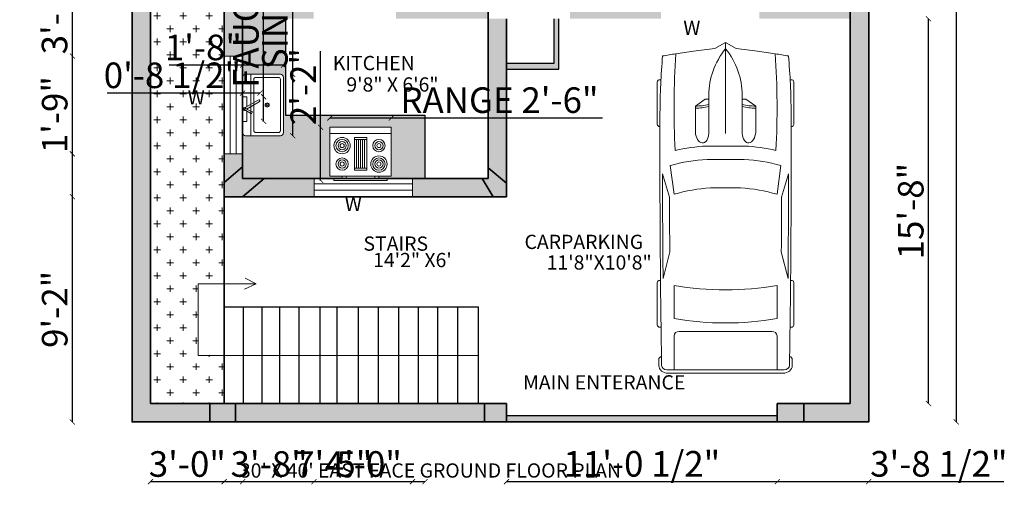
# Model space of a CAD drawing. Units: inches. Extents: x 1858 to 2399, y 1317 to 1943.
# Tile 1 of 8: x 1858 to 2340, y 1317 to 1554. Entities that reach past the tile are written whole.
import ezdxf

# ---------------------------------------------------------------- set-up
doc = ezdxf.new("R2010")
doc.units = ezdxf.units.IN
for name, color, linetype, lineweight in [('A-ANNO-DIMS', 2, 'Continuous', 18), ('A-ANNO-SYMB', 7, 'Continuous', 18), ('A-ANNO-TEXT', 7, 'Continuous', 18), ('A-AREA-IDEN', 7, 'Continuous', 18), ('A-COLS', 7, 'Continuous', 35), ('A-COLS-PATT', 5, 'Continuous', 13), ('A-DOOR', 4, 'Continuous', 25), ('A-EQPM', 8, 'Continuous', 18), ('A-EQPM-VEHI', 8, 'Continuous', 18), ('A-FLOR-CASE', 8, 'Continuous', 25), ('A-FLOR-FIXT', 9, 'Continuous', 18), ('A-FLOR-FIXT-PATT', 9, 'Continuous', 13), ('A-WALL', 7, 'Continuous', 35), ('A-WALL-PATT', 1, 'Continuous', 13), ('L-SITE-PATT', 8, 'Continuous', 13), ('stairs', 3, 'Continuous', 25), ('window', 4, 'Continuous', 18)]:
    doc.layers.add(name, color=color, linetype=linetype, lineweight=lineweight)
doc.styles.get("Standard").update_dxf_attribs({"font": 'arial.ttf'})
doc.dimstyles.new('ISO-25', dxfattribs={"dimtxt": 12.5, "dimasz": 2.5, "dimexe": 1.25, "dimexo": 0.625, "dimtad": 1, "dimdec": 0, "dimlunit": 4, "dimtxsty": 'Standard', "dimblk": 'ARCHTICK', "dimcen": 2.5, "dimse1": 1, "dimse2": 1, "dimclrd": 3, "dimclrt": 4, "dimadec": 0, "dimazin": 0, "dimtfac": 1, "dimtdec": 0, "dimtmove": 0, "dimatfit": 3, "dimfxl": 1, "dimarcsym": 0})

# ---------------------------------------------------------------- blocks, each defined once
blk = doc.blocks.new('*U6')
for p, q in [((21.1, 37.41), (21.1, 36.83)), ((46.55, 38.89), (22.35, 38.89)), ((47.8, 37.39), (47.8, 37.41)), ((87.99, 31.87), (74.76, 35.92)), ((134.31, 35.6), (119.29, 31.78)), ((135.45, 37.07), (135.45, 37.41)), ((136.7, 38.89), (160.9, 38.89)), ((162.15, 37.41), (162.15, 36.77)), ((70.03, 31.54), (86.41, 29.35)), ((138.42, 29.35), (157.25, 29.35)), ((186.47, 29.35), (167.01, 29.35)), ((186.47, -33.5), (186.47, 33.5)), ((188.4, -32.76), (188.4, 32.76)), ((164.52, 26.39), (164.52, -26.39)), ((32.27, 11.63), (36.13, 17.17)), ((36.13, 17.17), (50.94, 17.17)), ((3.27, 6.13), (0.1, 0.41)), ((29.77, 9.51), (51.68, 9.51)), ((32.12, 9.51), (32.12, 11.15)), ((58.92, -10.77), (58.92, 10.77)), ((66.55, -10.53), (66.55, 10.53)), ((82.74, 8.5), (82.74, -8.5)), ((186.47, -10.53), (186.47, 10.53)), ((0, 0), (51.68, 0)), ((0.1, -0.41), (3.27, -6.13)), ((29.77, -9.51), (51.68, -9.51)), ((32.12, -9.51), (32.12, -11.15)), ((32.27, -11.63), (36.13, -17.17)), ((36.13, -17.17), (50.94, -17.17)), ((86.41, -29.35), (70.03, -31.54)), ((87.99, -31.87), (74.76, -35.92)), ((134.31, -35.6), (119.29, -31.78)), ((157.25, -29.35), (138.42, -29.35)), ((167.01, -29.35), (186.47, -29.35)), ((21.1, -37.41), (21.1, -36.83)), ((46.55, -38.89), (22.35, -38.89)), ((47.8, -37.39), (47.8, -37.41)), ((135.45, -37.07), (135.45, -37.41)), ((136.7, -38.89), (160.9, -38.89)), ((162.15, -37.41), (162.15, -36.77))]:
    blk.add_line(p, q)
for centre, major_axis, ratio, start_param, end_param in [((266.03, -27.52), (0, 313.31), 0.842304, 1.367076, 1.39176), ((41.19, -490.86), (0, 528.23), 0.842304, 0.00281, 0.075598), ((22.35, 37.41), (0, -1.48), 0.842304, 3.141593, 4.712389), ((64.48, -10555.62), (0, 10593.03), 0.842304, -0.013397, 0.002797), ((46.55, 37.41), (0, 1.48), 0.842304, -1.570796, 0), ((64.48, -10555.62), (0, -10591.55), 0.842304, 3.133765, 3.140441), ((136.7, 37.41), (0, -1.48), 0.842304, 3.141593, 4.712389), ((160.9, 37.41), (0, 1.48), 0.842304, -1.570796, 0), ((180.63, 35.84), (0, 2.22), 0.842304, -0.013017, 1.249894), ((64.48, -10556.36), (0, 10595.31), 0.842304, -0.013397, -0.013017), ((183.98, 33.5), (0, -2.96), 0.842304, 1.570796, 3.128196), ((183.98, 32.76), (0, -5.25), 0.842304, 1.570796, 3.128196), ((259.18, -27.52), (0, -305.3), 0.842304, 4.528606, 4.561838), ((37.47, -593.96), (0, -623.33), 0.842304, 3.096046, 3.200911), ((134.4, 5.39), (0, -89.78), 0.842304, 4.449482, 4.652344), ((135.29, 5.39), (0, 81.77), 0.842304, 1.245306, 1.50788), ((149.6, 2.8), (0, -79.58), 0.842304, 4.372215, 4.640744), ((95.79, -3666.35), (0, -3698.24), 0.842304, 3.134049, 3.144098), ((17.08, 0), (0, 147.02), 0.842304, 4.511394, 4.913384), ((35.91, 0), (0, 147.02), 0.842304, 4.511394, 4.913384), ((167.01, 26.39), (0, 2.96), 0.842304, 0, 1.570796), ((-204.49, 52.4), (0, -250.96), 0.842304, 1.385369, 1.434372), ((13.04, 17.01), (0, 27.42), 0.842304, 4.435146, 4.718221), ((14.2, 17.01), (0, 27.42), 0.842304, 4.435146, 4.718221), ((50.79, 13.34), (6.34, -0.36), 0.603834, -1.395552, 1.581315), ((32.75, 11.15), (0, 0.74), 0.842304, 0.879714, 1.570796), ((29.77, -46.66), (0, 56.17), 0.842304, 0, 0.590319), ((0.62, 0), (0, -0.74), 0.842304, 4.131459, 5.293319), ((29.77, 46.66), (0, 56.17), 0.842304, 2.551274, 3.141593), ((-204.49, -52.4), (0, 250.96), 0.842304, -1.434372, -1.385369), ((32.75, -11.15), (0, -0.74), 0.842304, 4.712389, 5.403472), ((13.04, -17.01), (0, -27.42), 0.842304, 1.564964, 1.848039), ((14.2, -17.01), (0, -27.42), 0.842304, 1.564964, 1.848039), ((134.4, -5.39), (0, -89.78), 0.842304, -1.510751, -1.307889), ((135.29, -5.39), (0, -81.77), 0.842304, -1.50788, -1.245306), ((149.6, -2.8), (0, -79.58), 0.842304, -1.499151, -1.230623), ((259.18, 27.52), (0, 305.3), 0.842304, 1.721348, 1.754579), ((167.01, -26.39), (0, -2.96), 0.842304, 4.712389, 6.283185), ((266.03, 27.52), (0, 313.31), 0.842304, 1.749832, 1.774517), ((37.47, 593.96), (0, -623.33), 0.842304, -0.059319, 0.045547), ((95.79, 3666.35), (0, -3698.24), 0.842304, -0.002505, 0.007544), ((183.98, -33.5), (0, 2.96), 0.842304, 3.15499, 4.712389), ((183.98, -32.76), (0, -5.25), 0.842304, 0.013397, 1.570796), ((41.19, 490.86), (0, -528.23), 0.842304, -0.075598, -0.00281), ((22.35, -37.41), (0, 1.48), 0.842304, 1.570796, 3.141593), ((64.48, 10555.62), (0, 10593.03), 0.842304, 3.138796, 3.15499), ((46.55, -37.41), (0, -1.48), 0.842304, 0, 1.570796), ((64.48, 10555.62), (0, -10591.55), 0.842304, 0.001152, 0.007828), ((136.7, -37.41), (0, -1.48), 0.842304, -1.570796, 0), ((160.9, -37.41), (0, 1.48), 0.842304, 3.141593, 4.712389), ((180.63, -35.84), (0, -2.22), 0.842304, -1.249894, 0.013017), ((64.48, 10556.36), (0, 10595.31), 0.842304, 3.15461, 3.15499)]:
    blk.add_ellipse(centre, major_axis=major_axis, ratio=ratio, start_param=start_param, end_param=end_param)
at = {"extrusion": (0, 0, -1)}
blk.add_ellipse((50.79, -13.34), major_axis=(6.34, 0.36), ratio=0.603834, start_param=-1.395552, end_param=1.581315, dxfattribs=at)
blk = doc.blocks.new('Range-Oven - 30 in top')
for p, q in [((0, -3), (30, -3)), ((12, -6), (18, -6)), ((13, -20), (13, -6)), ((14, -6), (14, -20)), ((15, -20), (15, -6)), ((16, -6), (16, -20)), ((17, -20), (17, -6)), ((6, -24), (6, -25)), ((8, -25), (8, -24)), ((18, -20), (12, -20)), ((22, -25), (22, -24)), ((24, -24), (24, -25))]:
    blk.add_line(p, q)
for points in [[(0, -24), (0, 0), (30, 0), (30, -24)], [(12, -21), (12, -5), (18, -5), (18, -21)], [(2, -26), (2, -25), (28, -25), (28, -26)]]:
    blk.add_lwpolyline(points, close=True)
for centre, radius in [((6, -9), 4), ((6, -9), 3), ((6, -9), 2), ((6, -9), 1), ((24, -9), 3), ((24, -9), 2), ((24, -9), 1), ((24, -18), 4), ((6, -18), 3), ((6, -18), 2), ((6, -18), 1), ((24, -18), 3), ((24, -18), 2), ((24, -18), 1)]:
    blk.add_circle(centre, radius)
blk = doc.blocks.new('Sink-single - 30 in top')
blk.add_line((-15, -3.999996), (15, -3.999996))
for points in [[(-13.5, 0), (13.5, 0)], [(-15, -18.499996), (-15, -1.5)], [(15, -1.5), (15, -18.499996)], [(-13.5, -17.499996), (-13.5, -6.499996)], [(-12.5, -5.499996), (12.5, -5.499996)], [(13.5, -6.499996), (13.5, -17.499996)], [(12.5, -18.499996), (-12.5, -18.499996)], [(13.5, -19.999996), (-13.5, -19.999996)]]:
    blk.add_lwpolyline(points)
for radius in [1, 0.5]:
    blk.add_circle((0, -11.999996), radius)
for centre, radius, start, end in [((-13.5, -1.5), 1.5, 90, 180), ((13.5, -1.5), 1.5, 0, 90), ((-12.5, -6.499996), 1, 90, 180), ((12.5, -6.499996), 1, 0, 90), ((-13.5, -18.499996), 1.5, 180, 270), ((-12.5, -17.499996), 1, 180, 270), ((12.5, -17.499996), 1, 270, 0), ((13.5, -18.499996), 1.5, 270, 0)]:
    blk.add_arc(centre, radius, start, end)
blk = doc.blocks.new('Faucet - single handle top')
for p, q in [((0.08, -0.26), (-2.26, -4.34)), ((-2.26, -4.34), (-1.37, -4.79)), ((-1.37, -4.79), (0.55, -0.5)), ((-0.06, -1.9), (3.57, -8.18)), ((4.43, -7.68), (0.72, -1.24))]:
    blk.add_line(p, q)
for points in [[(-0.92, -2), (-6, -2), (-6, 0), (6, 0), (6, -2), (1.16, -2)], [(-0.01, -2), (-0.12, -2)]]:
    blk.add_lwpolyline(points)
for centre, radius, start, end in [((0, -1), 0.75, 269.2246, 216.2304), ((4, -7.93), 0.5, 210, 30)]:
    blk.add_arc(centre, radius, start, end)
blk = doc.blocks.new('_ArchTick')
at = {"color": 0, "linetype": 'ByBlock', "const_width": 0.15}
blk.add_lwpolyline([(-0.5, -0.5), (0.5, 0.5)], dxfattribs=at)
blk = doc.blocks.new('*D13')
at = {"layer": 'A-ANNO-DIMS', "color": 0, "lineweight": -2, "transparency": 16777216}
blk.add_line((2316.13, 1837.34), (2316.13, 1357.34), dxfattribs=at)
at = {"layer": 'Defpoints', "color": 0, "transparency": 16777216}
for p in [(2273.38, 1837.34), (2273.38, 1357.34), (2316.13, 1357.34)]:
    blk.add_point(p, dxfattribs=at)
at = {"layer": 'A-ANNO-DIMS', "color": 0, "lineweight": -2, "transparency": 16777216, "xscale": 2.5, "yscale": 2.5, "zscale": 2.5}
for p, rotation in [((2316.13, 1837.34), 90), ((2316.13, 1357.34), 270)]:
    blk.add_blockref('_ArchTick', p, dxfattribs=dict(at, rotation=rotation))
at = {"layer": 'A-ANNO-DIMS', "color": 0, "transparency": 16777216, "insert": (2309.12, 1597.34), "char_height": 12.5, "attachment_point": 5, "rotation": 90}
blk.add_mtext("40'", dxfattribs=at)
blk = doc.blocks.new('*D19')
at = {"layer": 'A-ANNO-DIMS', "color": 3, "lineweight": -2, "transparency": 16777216}
for p, q in [((2010.03, 1505.84), (2040.03, 1505.84)), ((2040.03, 1505.84), (2143.31, 1505.84))]:
    blk.add_line(p, q, dxfattribs=at)
at = {"layer": 'Defpoints', "color": 0, "transparency": 16777216}
for p in [(2040.03, 1505.84), (2010.03, 1501.34), (2040.03, 1501.34)]:
    blk.add_point(p, dxfattribs=at)
at = {"layer": 'A-ANNO-DIMS', "color": 3, "lineweight": -2, "transparency": 16777216, "xscale": 2.5, "yscale": 2.5, "zscale": 2.5, "rotation": 180}
blk.add_blockref('_ArchTick', (2010.03, 1505.84), dxfattribs=at)
at = {"layer": 'A-ANNO-DIMS', "color": 3, "lineweight": -2, "transparency": 16777216, "xscale": 2.5, "yscale": 2.5, "zscale": 2.5}
blk.add_blockref('_ArchTick', (2040.03, 1505.84), dxfattribs=at)
at = {"layer": 'A-ANNO-DIMS', "color": 4, "transparency": 16777216, "insert": (2092.92, 1512.93), "char_height": 12.5, "attachment_point": 5}
blk.add_mtext('RANGE 2\'-6"', dxfattribs=at)
blk = doc.blocks.new('*D20')
at = {"layer": 'A-ANNO-DIMS', "color": 3, "lineweight": -2, "transparency": 16777216}
for p, q in [((2005.53, 1501.34), (2005.53, 1538.53)), ((2005.53, 1475.34), (2005.53, 1501.34))]:
    blk.add_line(p, q, dxfattribs=at)
at = {"layer": 'Defpoints', "color": 0, "transparency": 16777216}
for p in [(2005.53, 1501.34), (2010.03, 1501.34), (2010.03, 1475.34)]:
    blk.add_point(p, dxfattribs=at)
at = {"layer": 'A-ANNO-DIMS', "color": 3, "lineweight": -2, "transparency": 16777216, "xscale": 2.5, "yscale": 2.5, "zscale": 2.5}
for p, rotation in [((2005.53, 1501.34), 90), ((2005.53, 1475.34), 270)]:
    blk.add_blockref('_ArchTick', p, dxfattribs=dict(at, rotation=rotation))
at = {"layer": 'A-ANNO-DIMS', "color": 4, "transparency": 16777216, "insert": (1998.63, 1521.19), "char_height": 12.5, "attachment_point": 5, "rotation": 90}
blk.add_mtext('2\'-2"', dxfattribs=at)
blk = doc.blocks.new('*D21')
at = {"layer": 'A-ANNO-DIMS', "color": 3, "lineweight": -2, "transparency": 16777216}
for p, q in [((1991.88, 1527.2), (1991.88, 1609.72)), ((1991.88, 1497.2), (1991.88, 1527.2))]:
    blk.add_line(p, q, dxfattribs=at)
at = {"layer": 'Defpoints', "color": 0, "transparency": 16777216}
for p in [(1987.38, 1527.2), (1991.88, 1527.2), (1987.38, 1497.2)]:
    blk.add_point(p, dxfattribs=at)
at = {"layer": 'A-ANNO-DIMS', "color": 3, "lineweight": -2, "transparency": 16777216, "xscale": 2.5, "yscale": 2.5, "zscale": 2.5}
for p, rotation in [((1991.88, 1527.2), 90), ((1991.88, 1497.2), 270)]:
    blk.add_blockref('_ArchTick', p, dxfattribs=dict(at, rotation=rotation))
at = {"layer": 'A-ANNO-DIMS', "color": 4, "transparency": 16777216, "insert": (1984.79, 1569.71), "char_height": 12.5, "attachment_point": 5, "rotation": 90}
blk.add_mtext('SINK 2\'-6"', dxfattribs=at)
blk = doc.blocks.new('*D22')
at = {"layer": 'A-ANNO-DIMS', "color": 3, "lineweight": -2, "transparency": 16777216}
for p, q in [((1967.38, 1531.7), (1931.57, 1531.7)), ((1987.38, 1531.7), (1967.38, 1531.7))]:
    blk.add_line(p, q, dxfattribs=at)
at = {"layer": 'Defpoints', "color": 0, "transparency": 16777216}
for p in [(1967.38, 1531.7), (1967.38, 1527.2), (1987.38, 1527.2)]:
    blk.add_point(p, dxfattribs=at)
at = {"layer": 'A-ANNO-DIMS', "color": 3, "lineweight": -2, "transparency": 16777216, "xscale": 2.5, "yscale": 2.5, "zscale": 2.5, "rotation": 180}
blk.add_blockref('_ArchTick', (1967.38, 1531.7), dxfattribs=at)
at = {"layer": 'A-ANNO-DIMS', "color": 3, "lineweight": -2, "transparency": 16777216, "xscale": 2.5, "yscale": 2.5, "zscale": 2.5}
blk.add_blockref('_ArchTick', (1987.38, 1531.7), dxfattribs=at)
at = {"layer": 'A-ANNO-DIMS', "color": 4, "transparency": 16777216, "insert": (1948.23, 1538.7), "char_height": 12.5, "attachment_point": 5}
blk.add_mtext('1\'-8"', dxfattribs=at)
blk = doc.blocks.new('*D23')
at = {"layer": 'A-ANNO-DIMS', "color": 3, "lineweight": -2, "transparency": 16777216}
for p, q in [((1977.68, 1516.18), (1977.68, 1627.15)), ((1977.68, 1504.18), (1977.68, 1516.18))]:
    blk.add_line(p, q, dxfattribs=at)
at = {"layer": 'Defpoints', "color": 0, "transparency": 16777216}
for p in [(1975.88, 1516.18), (1977.68, 1516.18), (1975.88, 1504.18)]:
    blk.add_point(p, dxfattribs=at)
at = {"layer": 'A-ANNO-DIMS', "color": 3, "lineweight": -2, "transparency": 16777216, "xscale": 2.5, "yscale": 2.5, "zscale": 2.5}
for p, rotation in [((1977.68, 1516.18), 90), ((1977.68, 1504.18), 270)]:
    blk.add_blockref('_ArchTick', p, dxfattribs=dict(at, rotation=rotation))
at = {"layer": 'A-ANNO-DIMS', "color": 4, "transparency": 16777216, "insert": (1970.59, 1572.91), "char_height": 12.5, "attachment_point": 5, "rotation": 90}
blk.add_mtext('FAUCET 1\'-0"', dxfattribs=at)
blk = doc.blocks.new('*D24')
at = {"layer": 'A-ANNO-DIMS', "color": 3, "lineweight": -2, "transparency": 16777216}
for p, q in [((1967.38, 1517.98), (1901.27, 1517.98)), ((1975.88, 1517.98), (1967.38, 1517.98))]:
    blk.add_line(p, q, dxfattribs=at)
at = {"layer": 'Defpoints', "color": 0, "transparency": 16777216}
for p in [(1967.38, 1517.98), (1967.38, 1516.18), (1975.88, 1516.18)]:
    blk.add_point(p, dxfattribs=at)
at = {"layer": 'A-ANNO-DIMS', "color": 3, "lineweight": -2, "transparency": 16777216, "xscale": 2.5, "yscale": 2.5, "zscale": 2.5, "rotation": 180}
blk.add_blockref('_ArchTick', (1967.38, 1517.98), dxfattribs=at)
at = {"layer": 'A-ANNO-DIMS', "color": 3, "lineweight": -2, "transparency": 16777216, "xscale": 2.5, "yscale": 2.5, "zscale": 2.5}
blk.add_blockref('_ArchTick', (1975.88, 1517.98), dxfattribs=at)
at = {"layer": 'A-ANNO-DIMS', "color": 4, "transparency": 16777216, "insert": (1933.07, 1525.07), "char_height": 12.5, "attachment_point": 5}
blk.add_mtext('0\'-8 1/2"', dxfattribs=at)
blk = doc.blocks.new('*D25')
at = {"layer": 'A-ANNO-DIMS', "color": 3, "lineweight": -2, "transparency": 16777216}
for p, q in [((1993.57, 1565.17), (2036.62, 1565.17)), ((2036.62, 1565.17), (2177.76, 1565.17))]:
    blk.add_line(p, q, dxfattribs=at)
at = {"layer": 'Defpoints', "color": 0, "transparency": 16777216}
for p in [(1993.57, 1571.63), (2036.62, 1571.63), (2036.62, 1565.17)]:
    blk.add_point(p, dxfattribs=at)
at = {"layer": 'A-ANNO-DIMS', "color": 3, "lineweight": -2, "transparency": 16777216, "xscale": 2.5, "yscale": 2.5, "zscale": 2.5, "rotation": 180}
blk.add_blockref('_ArchTick', (1993.57, 1565.17), dxfattribs=at)
at = {"layer": 'A-ANNO-DIMS', "color": 3, "lineweight": -2, "transparency": 16777216, "xscale": 2.5, "yscale": 2.5, "zscale": 2.5}
blk.add_blockref('_ArchTick', (2036.62, 1565.17), dxfattribs=at)
at = {"layer": 'A-ANNO-DIMS', "color": 4, "transparency": 16777216, "insert": (2108.44, 1572.26), "char_height": 12.5, "attachment_point": 5}
blk.add_mtext('DINING SET 3\'-7"', dxfattribs=at)
blk = doc.blocks.new('*D28')
at = {"layer": 'A-ANNO-DIMS', "color": 3, "lineweight": -2, "transparency": 16777216}
blk.add_line((2096.38, 1328.14), (2228.69, 1328.14), dxfattribs=at)
at = {"layer": 'Defpoints', "color": 0, "transparency": 16777216}
for p in [(2096.38, 1360.3), (2228.69, 1360.3), (2228.69, 1328.14)]:
    blk.add_point(p, dxfattribs=at)
at = {"layer": 'A-ANNO-DIMS', "color": 3, "lineweight": -2, "transparency": 16777216, "xscale": 2.5, "yscale": 2.5, "zscale": 2.5, "rotation": 180}
blk.add_blockref('_ArchTick', (2096.38, 1328.14), dxfattribs=at)
at = {"layer": 'A-ANNO-DIMS', "color": 3, "lineweight": -2, "transparency": 16777216, "xscale": 2.5, "yscale": 2.5, "zscale": 2.5}
blk.add_blockref('_ArchTick', (2228.69, 1328.14), dxfattribs=at)
at = {"layer": 'A-ANNO-DIMS', "color": 4, "transparency": 16777216, "insert": (2162.53, 1335.23), "char_height": 12.5, "attachment_point": 5}
blk.add_mtext('11\'-0 1/2"', dxfattribs=at)
blk = doc.blocks.new('*D29')
at = {"layer": 'A-ANNO-DIMS', "color": 3, "lineweight": -2, "transparency": 16777216}
blk.add_line((2302.58, 1366.34), (2302.58, 1554.34), dxfattribs=at)
at = {"layer": 'Defpoints', "color": 0, "transparency": 16777216}
for p in [(2264.38, 1554.34), (2302.58, 1554.34), (2264.38, 1366.34)]:
    blk.add_point(p, dxfattribs=at)
at = {"layer": 'A-ANNO-DIMS', "color": 3, "lineweight": -2, "transparency": 16777216, "xscale": 2.5, "yscale": 2.5, "zscale": 2.5}
for p, rotation in [((2302.58, 1554.34), 90), ((2302.58, 1366.34), 270)]:
    blk.add_blockref('_ArchTick', p, dxfattribs=dict(at, rotation=rotation))
at = {"layer": 'A-ANNO-DIMS', "color": 4, "transparency": 16777216, "insert": (2295.57, 1460.34), "char_height": 12.5, "attachment_point": 5, "rotation": 90}
blk.add_mtext('15\'-8"', dxfattribs=at)
blk = doc.blocks.new('*D30')
at = {"layer": 'A-ANNO-DIMS', "color": 3, "lineweight": -2, "transparency": 16777216}
blk.add_line((1967.38, 1328.14), (2056.5, 1328.14), dxfattribs=at)
at = {"layer": 'Defpoints', "color": 0, "transparency": 16777216}
for p in [(1967.38, 1476.34), (2056.5, 1476.34), (2056.5, 1328.14)]:
    blk.add_point(p, dxfattribs=at)
at = {"layer": 'A-ANNO-DIMS', "color": 3, "lineweight": -2, "transparency": 16777216, "xscale": 2.5, "yscale": 2.5, "zscale": 2.5, "rotation": 180}
blk.add_blockref('_ArchTick', (1967.38, 1328.14), dxfattribs=at)
at = {"layer": 'A-ANNO-DIMS', "color": 3, "lineweight": -2, "transparency": 16777216, "xscale": 2.5, "yscale": 2.5, "zscale": 2.5}
blk.add_blockref('_ArchTick', (2056.5, 1328.14), dxfattribs=at)
at = {"layer": 'A-ANNO-DIMS', "color": 4, "transparency": 16777216, "insert": (2011.94, 1335.12), "char_height": 12.5, "attachment_point": 5}
blk.add_mtext('7\'-5"', dxfattribs=at)
blk = doc.blocks.new('*D39')
at = {"layer": 'A-ANNO-DIMS', "color": 3, "lineweight": -2, "transparency": 16777216}
for p, q in [((1884.18, 1488.33), (1884.18, 1524.13)), ((1884.18, 1467.34), (1884.18, 1488.33))]:
    blk.add_line(p, q, dxfattribs=at)
at = {"layer": 'Defpoints', "color": 0, "transparency": 16777216}
for p in [(1884.18, 1488.33), (1958.38, 1488.33), (1958.38, 1467.34)]:
    blk.add_point(p, dxfattribs=at)
at = {"layer": 'A-ANNO-DIMS', "color": 3, "lineweight": -2, "transparency": 16777216, "xscale": 2.5, "yscale": 2.5, "zscale": 2.5}
for p, rotation in [((1884.18, 1488.33), 90), ((1884.18, 1467.34), 270)]:
    blk.add_blockref('_ArchTick', p, dxfattribs=dict(at, rotation=rotation))
at = {"layer": 'A-ANNO-DIMS', "color": 4, "transparency": 16777216, "insert": (1877.17, 1507.48), "char_height": 12.5, "attachment_point": 5, "rotation": 90}
blk.add_mtext('1\'-9"', dxfattribs=at)
blk = doc.blocks.new('*D40')
at = {"layer": 'A-ANNO-DIMS', "color": 3, "lineweight": -2, "transparency": 16777216}
for p, q in [((1884.18, 1536.07), (1884.18, 1611.87)), ((1884.18, 1488.33), (1884.18, 1536.07))]:
    blk.add_line(p, q, dxfattribs=at)
at = {"layer": 'Defpoints', "color": 0, "transparency": 16777216}
for p in [(1884.18, 1536.07), (1958.38, 1536.07), (1958.38, 1488.33)]:
    blk.add_point(p, dxfattribs=at)
at = {"layer": 'A-ANNO-DIMS', "color": 3, "lineweight": -2, "transparency": 16777216, "xscale": 2.5, "yscale": 2.5, "zscale": 2.5}
for p, rotation in [((1884.18, 1536.07), 90), ((1884.18, 1488.33), 270)]:
    blk.add_blockref('_ArchTick', p, dxfattribs=dict(at, rotation=rotation))
at = {"layer": 'A-ANNO-DIMS', "color": 4, "transparency": 16777216, "insert": (1877.08, 1575.22), "char_height": 12.5, "attachment_point": 5, "rotation": 90}
blk.add_mtext('3\'-11 1/2"', dxfattribs=at)
blk = doc.blocks.new('*D41')
at = {"layer": 'A-ANNO-DIMS', "color": 3, "lineweight": -2, "transparency": 16777216}
for p, q in [((1884.18, 1591.74), (1884.18, 1658.34)), ((1884.18, 1536.07), (1884.18, 1591.74))]:
    blk.add_line(p, q, dxfattribs=at)
at = {"layer": 'Defpoints', "color": 0, "transparency": 16777216}
for p in [(1884.18, 1591.74), (1958.38, 1591.74), (1958.38, 1536.07)]:
    blk.add_point(p, dxfattribs=at)
at = {"layer": 'A-ANNO-DIMS', "color": 3, "lineweight": -2, "transparency": 16777216, "xscale": 2.5, "yscale": 2.5, "zscale": 2.5}
for p, rotation in [((1884.18, 1591.74), 90), ((1884.18, 1536.07), 270)]:
    blk.add_blockref('_ArchTick', p, dxfattribs=dict(at, rotation=rotation))
at = {"layer": 'A-ANNO-DIMS', "color": 4, "transparency": 16777216, "insert": (1877.09, 1626.29), "char_height": 12.5, "attachment_point": 5, "rotation": 90}
blk.add_mtext('4\'-7 1/2"', dxfattribs=at)
blk = doc.blocks.new('*D48')
at = {"layer": 'A-ANNO-DIMS', "color": 3, "lineweight": -2, "transparency": 16777216}
blk.add_line((1958.38, 1328.14), (2002.33, 1328.14), dxfattribs=at)
at = {"layer": 'Defpoints', "color": 0, "transparency": 16777216}
for p in [(1958.38, 1467.34), (2002.33, 1467.34), (2002.33, 1328.14)]:
    blk.add_point(p, dxfattribs=at)
at = {"layer": 'A-ANNO-DIMS', "color": 3, "lineweight": -2, "transparency": 16777216, "xscale": 2.5, "yscale": 2.5, "zscale": 2.5, "rotation": 180}
blk.add_blockref('_ArchTick', (1958.38, 1328.14), dxfattribs=at)
at = {"layer": 'A-ANNO-DIMS', "color": 3, "lineweight": -2, "transparency": 16777216, "xscale": 2.5, "yscale": 2.5, "zscale": 2.5}
blk.add_blockref('_ArchTick', (2002.33, 1328.14), dxfattribs=at)
at = {"layer": 'A-ANNO-DIMS', "color": 4, "transparency": 16777216, "insert": (1980.36, 1335.15), "char_height": 12.5, "attachment_point": 5}
blk.add_mtext('3\'-8"', dxfattribs=at)
blk = doc.blocks.new('*D49')
at = {"layer": 'A-ANNO-DIMS', "color": 3, "lineweight": -2, "transparency": 16777216}
blk.add_line((2002.33, 1328.14), (2050.44, 1328.14), dxfattribs=at)
at = {"layer": 'Defpoints', "color": 0, "transparency": 16777216}
for p in [(2002.33, 1467.34), (2050.44, 1467.34), (2050.44, 1328.14)]:
    blk.add_point(p, dxfattribs=at)
at = {"layer": 'A-ANNO-DIMS', "color": 3, "lineweight": -2, "transparency": 16777216, "xscale": 2.5, "yscale": 2.5, "zscale": 2.5, "rotation": 180}
blk.add_blockref('_ArchTick', (2002.33, 1328.14), dxfattribs=at)
at = {"layer": 'A-ANNO-DIMS', "color": 3, "lineweight": -2, "transparency": 16777216, "xscale": 2.5, "yscale": 2.5, "zscale": 2.5}
blk.add_blockref('_ArchTick', (2050.44, 1328.14), dxfattribs=at)
at = {"layer": 'A-ANNO-DIMS', "color": 4, "transparency": 16777216, "insert": (2026.39, 1335.15), "char_height": 12.5, "attachment_point": 5}
blk.add_mtext('4\'-0"', dxfattribs=at)
blk = doc.blocks.new('*D53')
at = {"layer": 'A-ANNO-DIMS', "color": 3, "lineweight": -2, "transparency": 16777216}
blk.add_line((1884.18, 1357.34), (1884.18, 1467.34), dxfattribs=at)
at = {"layer": 'Defpoints', "color": 0, "transparency": 16777216}
for p in [(1884.18, 1467.34), (1958.38, 1467.34), (1913.38, 1357.34)]:
    blk.add_point(p, dxfattribs=at)
at = {"layer": 'A-ANNO-DIMS', "color": 3, "lineweight": -2, "transparency": 16777216, "xscale": 2.5, "yscale": 2.5, "zscale": 2.5}
for p, rotation in [((1884.18, 1467.34), 90), ((1884.18, 1357.34), 270)]:
    blk.add_blockref('_ArchTick', p, dxfattribs=dict(at, rotation=rotation))
at = {"layer": 'A-ANNO-DIMS', "color": 4, "transparency": 16777216, "insert": (1877.17, 1412.34), "char_height": 12.5, "attachment_point": 5, "rotation": 90}
blk.add_mtext('9\'-2"', dxfattribs=at)
blk = doc.blocks.new('*D54')
at = {"layer": 'A-ANNO-DIMS', "color": 3, "lineweight": -2, "transparency": 16777216}
blk.add_line((1922.38, 1328.14), (1958.38, 1328.14), dxfattribs=at)
at = {"layer": 'Defpoints', "color": 0, "transparency": 16777216}
for p in [(1922.38, 1366.34), (1958.38, 1366.34), (1958.38, 1328.14)]:
    blk.add_point(p, dxfattribs=at)
at = {"layer": 'A-ANNO-DIMS', "color": 3, "lineweight": -2, "transparency": 16777216, "xscale": 2.5, "yscale": 2.5, "zscale": 2.5, "rotation": 180}
blk.add_blockref('_ArchTick', (1922.38, 1328.14), dxfattribs=at)
at = {"layer": 'A-ANNO-DIMS', "color": 3, "lineweight": -2, "transparency": 16777216, "xscale": 2.5, "yscale": 2.5, "zscale": 2.5}
blk.add_blockref('_ArchTick', (1958.38, 1328.14), dxfattribs=at)
at = {"layer": 'A-ANNO-DIMS', "color": 4, "transparency": 16777216, "insert": (1940.38, 1335.15), "char_height": 12.5, "attachment_point": 5}
blk.add_mtext('3\'-0"', dxfattribs=at)
blk = doc.blocks.new('*D55')
at = {"layer": 'A-ANNO-DIMS', "color": 3, "lineweight": -2, "transparency": 16777216}
for p, q in [((2228.69, 1328.14), (2273.38, 1328.14)), ((2273.38, 1328.14), (2339.47, 1328.14))]:
    blk.add_line(p, q, dxfattribs=at)
at = {"layer": 'Defpoints', "color": 0, "transparency": 16777216}
for p in [(2228.69, 1360.3), (2273.38, 1357.34), (2273.38, 1328.14)]:
    blk.add_point(p, dxfattribs=at)
at = {"layer": 'A-ANNO-DIMS', "color": 3, "lineweight": -2, "transparency": 16777216, "xscale": 2.5, "yscale": 2.5, "zscale": 2.5, "rotation": 180}
blk.add_blockref('_ArchTick', (2228.69, 1328.14), dxfattribs=at)
at = {"layer": 'A-ANNO-DIMS', "color": 3, "lineweight": -2, "transparency": 16777216, "xscale": 2.5, "yscale": 2.5, "zscale": 2.5}
blk.add_blockref('_ArchTick', (2273.38, 1328.14), dxfattribs=at)
at = {"layer": 'A-ANNO-DIMS', "color": 4, "transparency": 16777216, "insert": (2307.67, 1335.23), "char_height": 12.5, "attachment_point": 5}
blk.add_mtext('3\'-8 1/2"', dxfattribs=at)

msp = doc.modelspace()

# ---------------------------------------------------------------- hatches: boundary and pattern name
at = {"layer": 'A-COLS-PATT'}
h = msp.add_hatch(color=256, dxfattribs=at)
h.dxf.hatch_style = 1
h.paths.add_polyline_path([(1977.99, 1696.34), (1967.38, 1696.34), (1967.38, 1700.89), (1958.38, 1700.89), (1958.38, 1685.05), (1967.38, 1685.05), (1967.38, 1691.34), (1977.99, 1691.34)])
h.paths.add_polyline_path([(1967.38, 1571.83), (1958.38, 1571.83), (1958.38, 1559.34), (1967.38, 1559.34)])
h.paths.add_polyline_path([(1977.97, 1476.34), (1967.38, 1476.34), (1967.38, 1482.01), (1958.38, 1474.25), (1958.38, 1467.34), (1967.38, 1467.34)])
h.paths.add_polyline_path([(2096.38, 1473.96), (2087.38, 1481.51), (2087.38, 1476.34), (2084.48, 1476.34), (2089.85, 1467.34), (2096.38, 1467.34)])
h.paths.add_polyline_path([(2273.38, 1837.34), (2265.79, 1837.34), (2258.24, 1828.34), (2264.38, 1828.34), (2264.38, 1823.36), (2273.38, 1827.14)])
h.paths.add_polyline_path([(2097.64, 1837.34), (2082.58, 1837.34), (2082.58, 1828.34), (2097.64, 1828.34)])
h.paths.add_polyline_path([(1977.66, 1837.34), (1949.42, 1837.34), (1949.42, 1828.34), (1977.66, 1828.34)])
h = msp.add_hatch(color=256, dxfattribs=at)
h.dxf.hatch_style = 1
h.paths.add_polyline_path([(2273.38, 1706.46), (2264.38, 1706.46), (2264.38, 1691.34), (2273.38, 1691.34)])
h.paths.add_polyline_path([(2273.38, 1576.35), (2264.38, 1576.35), (2264.38, 1563.34), (2273.38, 1563.34)])
h.paths.add_polyline_path([(2241.64, 1366.34), (2228.69, 1366.34), (2228.69, 1357.34), (2241.64, 1357.34)])
h.paths.add_polyline_path([(2096.38, 1366.34), (2085.57, 1366.34), (2085.57, 1357.34), (2096.38, 1357.34)])
h.paths.add_polyline_path([(1963.94, 1366.34), (1951.36, 1366.34), (1951.36, 1357.34), (1963.94, 1357.34)])
at = {"layer": 'A-FLOR-FIXT-PATT'}
h = msp.add_hatch(color=256, dxfattribs=at)
h.dxf.hatch_style = 1
h.set_gradient(color1=(0, 0, 255), color2=(255, 255, 0))
h.paths.add_polyline_path([(2010.03, 1501.34), (2040.03, 1501.34), (2040.03, 1477.34), (2034.03, 1477.34), (2034.03, 1476.34), (2038.03, 1476.34), (2050.44, 1476.34), (2056.5, 1476.34), (2056.5, 1507.28), (1988.35, 1507.28), (1988.35, 1554.34), (1967.38, 1554.34), (1967.38, 1525.7, -0.414214), (1968.88, 1527.2), (1985.88, 1527.2, -0.414214), (1987.38, 1525.7), (1987.38, 1498.7, -0.414214), (1985.88, 1497.2), (1968.88, 1497.2, -0.414214), (1967.38, 1498.7), (1967.38, 1476.34), (2016.03, 1476.34), (2016.03, 1477.34), (2010.03, 1477.34)])
h.paths.add_polyline_path([(2129, 1826.59, 0.414214), (2128, 1827.34), (2110.75, 1827.34, 0.414214), (2110, 1826.34), (2110, 1822.09, 0.414214), (2111, 1821.34), (2128.25, 1821.34, 0.414214), (2129, 1822.34)])
h.paths.add_polyline_path([(2047.65, 1651.34), (2026.65, 1651.34), (2026.65, 1643.34), (2047.65, 1643.34)])
h.paths.add_polyline_path([(2045.65, 1644.34, 0.5), (2046.65, 1645.34), (2046.65, 1649.34, 0.5), (2045.65, 1650.34), (2028.65, 1650.34, 0.5), (2027.65, 1649.34), (2027.65, 1645.34, 0.5), (2028.65, 1644.34)], flags=16)
at = {"layer": 'A-WALL-PATT'}
h = msp.add_hatch(color=256, dxfattribs=at)
h.dxf.hatch_style = 1
h.paths.add_polyline_path([(1967.38, 1742.58), (1958.38, 1742.58), (1958.38, 1700.89), (1967.38, 1700.89)])
h.paths.add_polyline_path([(1967.38, 1685.05), (1958.38, 1685.05), (1958.38, 1672.42), (1967.38, 1672.42)], flags=17)
h.paths.add_polyline_path([(2092.38, 1643.34), (2087.38, 1643.34), (2063.38, 1643.34), (2063.38, 1691.34), (2087.38, 1691.34), (2092.38, 1691.34), (2092.38, 1696.34), (2087.38, 1696.34), (2005.38, 1696.34), (2005.38, 1691.34), (2058.38, 1691.34), (2058.38, 1643.34), (1967.38, 1643.34), (1967.38, 1652.51), (1958.38, 1652.51), (1958.38, 1625.4), (1967.38, 1625.4), (1967.38, 1638.34), (2087.38, 1638.34), (2087.38, 1617.63), (2092.38, 1617.63)])
h.paths.add_polyline_path([(1967.38, 1591.74), (1958.38, 1591.74), (1958.38, 1571.83), (1967.38, 1571.83)])
h.paths.add_polyline_path([(1967.38, 1554.34), (2002.1, 1554.34), (2002.1, 1559.34), (1967.38, 1559.34), (1958.38, 1559.34), (1958.38, 1536.07), (1967.38, 1536.07)])
h.paths.add_polyline_path([(2087.38, 1559.34), (2042.3, 1559.34), (2042.3, 1554.34), (2087.38, 1554.34)])
h.paths.add_polyline_path([(2092.38, 1583.24), (2087.38, 1583.24), (2087.38, 1563.34), (2092.38, 1563.34)])
h.paths.add_polyline_path([(2096.38, 1554.34), (2087.38, 1554.34), (2087.38, 1481.51), (2096.38, 1473.96)])
h.paths.add_polyline_path([(2084.48, 1476.34), (2050.44, 1476.34), (2050.44, 1467.34), (2089.85, 1467.34)])
h.paths.add_polyline_path([(2002.33, 1476.34), (1977.97, 1476.34), (1967.38, 1467.34), (2002.33, 1467.34)])
h.paths.add_polyline_path([(1967.38, 1488.33), (1958.38, 1488.33), (1958.38, 1474.25), (1967.38, 1482.01)])
h.paths.add_polyline_path([(2121.99, 1554.34), (2119.71, 1554.34), (2119.71, 1532.61), (2096.38, 1532.61), (2096.38, 1529.65), (2121.99, 1529.65)])
h.paths.add_polyline_path([(2171.86, 1563.34), (2127.41, 1563.34), (2127.41, 1554.34), (2171.86, 1554.34)])
h.paths.add_polyline_path([(2264.38, 1563.34), (2220, 1563.34), (2220, 1554.34), (2264.38, 1554.34)])
h.paths.add_polyline_path([(2273.38, 1563.34), (2264.38, 1563.34), (2264.38, 1366.34), (2241.64, 1366.34), (2241.64, 1357.34), (2273.38, 1357.34)])
h.paths.add_polyline_path([(2273.38, 1691.34), (2264.38, 1691.34), (2264.38, 1576.35), (2273.38, 1576.35)])
h.paths.add_polyline_path([(2273.38, 1827.14), (2264.38, 1823.36), (2264.38, 1706.46), (2273.38, 1706.46)])
h.paths.add_polyline_path([(2265.79, 1837.34), (2234.56, 1837.34), (2234.56, 1828.34), (2258.24, 1828.34)])
h.paths.add_polyline_path([(2186.7, 1837.34), (2131.33, 1837.34), (2131.33, 1828.34), (2186.7, 1828.34)])
h.paths.add_polyline_path([(2107.67, 1837.34), (2097.64, 1837.34), (2097.64, 1828.34), (2107.67, 1828.34)])
h.paths.add_polyline_path([(2082.58, 1837.34), (2051.43, 1837.34), (2051.43, 1828.34), (2082.58, 1828.34)])
h.paths.add_polyline_path([(2092.38, 1828.34), (2087.38, 1828.34), (2087.38, 1729.93), (2092.38, 1729.93), (2092.38, 1739.34), (2140.38, 1739.34), (2140.38, 1730.57), (2145.38, 1730.57), (2145.38, 1828.34), (2140.38, 1828.34), (2140.38, 1744.34), (2092.38, 1744.34)])
h.paths.add_polyline_path([(1989.86, 1837.34), (1977.66, 1837.34), (1977.66, 1828.34), (1989.86, 1828.34)])
h.paths.add_polyline_path([(1922.38, 1822.27), (1913.38, 1826.41), (1913.38, 1357.34), (1951.36, 1357.34), (1951.36, 1366.34), (1922.38, 1366.34)])
h.paths.add_polyline_path([(1967.38, 1828.34), (1958.38, 1828.34), (1958.38, 1791.57), (1967.38, 1791.57)])
h = msp.add_hatch(color=256, dxfattribs=at)
h.dxf.hatch_style = 1
h.paths.add_polyline_path([(2085.57, 1366.34), (1963.94, 1366.34), (1963.94, 1357.34), (2085.57, 1357.34)])
h.paths.add_polyline_path([(2228.69, 1360.3), (2096.38, 1360.3), (2096.38, 1357.34), (2228.69, 1357.34)])
at = {"layer": 'L-SITE-PATT'}
h = msp.add_hatch(dxfattribs=at)
h.set_pattern_fill('CROSS', color=256)
h.paths.add_polyline_path([(1958.38, 1820.26), (1922.38, 1820.26), (1922.38, 1366.34), (1958.38, 1366.34), (1958.38, 1389.85), (1945.69, 1389.85), (1945.69, 1424.76), (1958.38, 1424.76)])
h.paths.add_polyline_path([(1943.89, 1763.53), (1956.55, 1763.53), (1956.55, 1773.97), (1943.89, 1773.97)], flags=24)
h.paths.add_polyline_path([(1948.35, 1662.61), (1958.32, 1662.61), (1958.32, 1673.05), (1948.35, 1673.05)], flags=24)
h.paths.add_polyline_path([(1938.82, 1510.71), (1951.47, 1510.71), (1951.47, 1521.15), (1938.82, 1521.15)], flags=24)
h.paths.add_polyline_path([(1939.14, 1601.55), (1951.8, 1601.55), (1951.8, 1611.99), (1939.14, 1611.99)], flags=24)

# ---------------------------------------------------------------- linework, layer by layer
at = {"layer": 'A-ANNO-SYMB'}
for p, q in [((1945.69, 1389.85), (1945.69, 1424.76)), ((1945.69, 1424.76), (1973.96, 1424.76)), ((1973.96, 1424.76), (1968.25, 1422.21)), ((1973.96, 1424.76), (1968.64, 1427.5)), ((1968.64, 1427.5), (1973.96, 1424.76)), ((2082.65, 1389.85), (1945.69, 1389.85))]:
    msp.add_line(p, q, dxfattribs=at)
at = {"layer": 'A-COLS'}
for p, q in [((1967.38, 1482.01), (1958.38, 1474.25)), ((2087.38, 1481.51), (2096.38, 1473.96)), ((1977.97, 1476.34), (1967.38, 1467.34)), ((2084.48, 1476.34), (2089.85, 1467.34)), ((1967.38, 1467.34), (1958.38, 1467.34)), ((1951.36, 1366.34), (1951.36, 1357.34)), ((1963.94, 1366.34), (1963.94, 1357.34)), ((2085.57, 1366.34), (2085.57, 1357.34)), ((2241.64, 1366.34), (2241.64, 1357.34))]:
    msp.add_line(p, q, dxfattribs=at)
at = {"layer": 'A-DOOR'}
msp.add_line((2228.69, 1360.3), (2096.38, 1360.3), dxfattribs=at)
at = {"layer": 'A-FLOR-CASE'}
for p, q in [((1988.35, 1554.34), (1988.35, 1507.28)), ((1988.35, 1507.28), (2056.5, 1507.28)), ((2056.5, 1507.28), (2056.5, 1476.34))]:
    msp.add_line(p, q, dxfattribs=at)
at = {"layer": 'A-WALL'}
for p, q in [((1958.38, 1366.34), (1958.38, 1828.34)), ((2264.38, 1828.34), (2264.38, 1366.34)), ((1922.38, 1366.34), (1922.38, 1822.27)), ((2087.38, 1476.34), (2087.38, 1583.24)), ((1967.38, 1476.34), (1967.38, 1554.34)), ((2096.38, 1467.34), (2096.38, 1554.34)), ((1967.38, 1476.34), (2087.38, 1476.34)), ((1967.38, 1467.34), (2096.38, 1467.34)), ((2096.38, 1366.34), (1922.38, 1366.34)), ((2096.38, 1366.34), (2096.38, 1357.34)), ((2264.38, 1366.34), (2228.69, 1366.34)), ((2228.69, 1366.34), (2228.69, 1357.34))]:
    msp.add_line(p, q, dxfattribs=at)
msp.add_lwpolyline([(1949.42, 1837.34), (2273.38, 1837.34), (2273.38, 1357.34), (1913.38, 1357.34), (1913.38, 1826.41)], dxfattribs=at)
at = {"layer": 'stairs'}
for p, q in [((2119.71, 1532.61), (2119.71, 1554.34)), ((2121.99, 1529.65), (2121.99, 1554.34)), ((2096.38, 1532.61), (2119.71, 1532.61)), ((2096.38, 1529.65), (2121.99, 1529.65)), ((1985.57, 1413.37), (1958.38, 1413.37)), ((1967.86, 1366.34), (1967.86, 1413.37)), ((1976.93, 1366.34), (1976.93, 1413.37)), ((1985.57, 1366.34), (1985.57, 1413.37)), ((2082.65, 1413.37), (1985.57, 1413.37)), ((1995.07, 1366.34), (1995.07, 1413.37)), ((2005.37, 1366.34), (2005.37, 1413.37)), ((2013.69, 1366.34), (2013.69, 1413.37)), ((2023.98, 1366.34), (2023.98, 1413.37)), ((2033.88, 1366.34), (2033.88, 1413.37)), ((2043.78, 1366.34), (2043.78, 1413.37)), ((2053.29, 1366.34), (2053.29, 1413.37)), ((2062.79, 1366.34), (2062.79, 1413.37)), ((2072.54, 1366.34), (2072.54, 1413.37)), ((2082.65, 1366.34), (2082.65, 1413.37))]:
    msp.add_line(p, q, dxfattribs=at)
at = {"layer": 'window'}
for p, q in [((1967.38, 1536.07), (1958.38, 1536.07)), ((1958.38, 1536.07), (1958.38, 1488.33)), ((1961.37, 1536.07), (1961.37, 1488.33)), ((1964.18, 1536.07), (1964.18, 1488.33)), ((1967.38, 1488.33), (1967.38, 1536.07)), ((1958.38, 1488.33), (1967.38, 1488.33)), ((2002.33, 1476.34), (2002.33, 1467.34)), ((2050.44, 1476.34), (2002.33, 1476.34)), ((2002.33, 1473.68), (2050.44, 1473.68)), ((2050.44, 1467.34), (2050.44, 1476.34)), ((2002.33, 1470.49), (2050.44, 1470.49)), ((2002.33, 1467.34), (2002.33, 1467.34)), ((2002.33, 1467.34), (2050.44, 1467.34))]:
    msp.add_line(p, q, dxfattribs=at)

# ---------------------------------------------------------------- block references
at = {"layer": 'A-EQPM'}
msp.add_blockref('Range-Oven - 30 in top', (2010.03, 1501.34), dxfattribs=at)
at = {"layer": 'A-EQPM-VEHI', "xscale": 0.8574523342081231, "yscale": 0.8574523342081231, "zscale": 0.8574523342081231, "rotation": 270}
msp.add_blockref('*U6', (2203.43, 1542.65), dxfattribs=at)
at = {"layer": 'A-FLOR-FIXT', "rotation": 90}
for name, p in [('Sink-single - 30 in top', (1967.38, 1512.2)), ('Faucet - single handle top', (1967.38, 1510.18))]:
    msp.add_blockref(name, p, dxfattribs=at)

# ---------------------------------------------------------------- texts
at = {"layer": 'A-ANNO-TEXT'}
for s, height, p in [('W', 6.96, (2182.79, 1546.43)), ('W', 6.96, (1940.56, 1512.45)), ('W', 6.96, (2017.33, 1460.37)), ('MAIN ENTERANCE', 6.9604, (2104.46, 1373.19)), ("30' X 40' EAST FACE GROUND FLOOR PLAN", 6.9604, (1966.07, 1330.12))]:
    msp.add_text(s, height=height, dxfattribs=at).set_placement(p)
at = {"layer": 'A-AREA-IDEN'}
for s, height, p in [('KITCHEN', 6.96, (2011.46, 1529.19)), ('9\'8" X 6\'6"', 6.9604, (2018.12, 1518.73)), ('CARPARKING', 6.96, (2105.17, 1441.83)), ('STAIRS', 6.96, (2026.46, 1440.98)), ('14\'2" X6\'', 6.96, (2031.19, 1432.95)), ('11\'8"X10\'8"', 6.9604, (2116, 1431.75))]:
    msp.add_text(s, height=height, dxfattribs=at).set_placement(p)

# ---------------------------------------------------------------- dimensions: what is measured, and where the dimension line sits
at = {"layer": 'A-ANNO-DIMS'}
for base, p1, p2, angle, override, picture, middle in [((2316.13, 1357.34), (2273.38, 1837.34), (2273.38, 1357.34), 90, {"dimclrd": 0, "dimclre": 0, "dimclrt": 0}, '*D13', (2309.12, 1597.34)), ((1884.18, 1591.74), (1958.38, 1536.07), (1958.38, 1591.74), 90, {"dimdec": 1, "dimlfac": 1, "dimrnd": 0, "dimzin": 1, "dimdsep": 46, "dimlunit": 4, "dimfrac": 2}, '*D41', (1877.09, 1626.29)), ((1884.18, 1536.07), (1958.38, 1488.33), (1958.38, 1536.07), 90, {"dimdec": 1, "dimlfac": 1, "dimrnd": 0, "dimzin": 1, "dimdsep": 46, "dimlunit": 4, "dimfrac": 2}, '*D40', (1877.08, 1575.22)), ((2302.58, 1554.34), (2264.38, 1366.34), (2264.38, 1554.34), 90, {"dimdec": 1, "dimlfac": 1, "dimrnd": 0, "dimzin": 1, "dimdsep": 46, "dimlunit": 4, "dimfrac": 2}, '*D29', (2295.57, 1460.34)), ((1967.38, 1531.7), (1987.38, 1527.2), (1967.38, 1527.2), 180, {"dimdec": 1, "dimlfac": 1, "dimrnd": 0, "dimzin": 1, "dimdsep": 46, "dimlunit": 4, "dimfrac": 2}, '*D22', (1948.23, 1538.7)), ((1967.38, 1517.98), (1975.88, 1516.18), (1967.38, 1516.18), 180, {"dimdec": 1, "dimlfac": 1, "dimrnd": 0, "dimzin": 1, "dimdsep": 46, "dimlunit": 4, "dimfrac": 2}, '*D24', (1933.07, 1525.07)), ((2005.53, 1501.34), (2010.03, 1475.34), (2010.03, 1501.34), 90, {"dimdec": 1, "dimlfac": 1, "dimrnd": 0, "dimzin": 1, "dimdsep": 46, "dimlunit": 4, "dimfrac": 2}, '*D20', (1998.63, 1521.19)), ((1884.18, 1488.33), (1958.38, 1467.34), (1958.38, 1488.33), 90, {"dimdec": 1, "dimlfac": 1, "dimrnd": 0, "dimzin": 1, "dimdsep": 46, "dimlunit": 4, "dimfrac": 2}, '*D39', (1877.17, 1507.48)), ((1884.18, 1467.34), (1913.38, 1357.34), (1958.38, 1467.34), 90, {"dimdec": 1, "dimlfac": 1, "dimrnd": 0, "dimzin": 1, "dimdsep": 46, "dimlunit": 4, "dimfrac": 2}, '*D53', (1877.17, 1412.34))]:
    dim = msp.add_linear_dim(base=base, p1=p1, p2=p2, angle=angle, dimstyle='ISO-25', override=override, dxfattribs=at)
    dim.commit()
    dim.dimension.update_dxf_attribs({"geometry": picture, "text_midpoint": middle})
for base, p1, p2, text, picture, middle in [((1977.68, 1516.18), (1975.88, 1504.18), (1975.88, 1516.18), 'FAUCET <>', '*D23', (1970.59, 1572.91)), ((1991.88, 1527.2), (1987.38, 1497.2), (1987.38, 1527.2), 'SINK <>', '*D21', (1984.79, 1569.71))]:
    dim = msp.add_linear_dim(base=base, p1=p1, p2=p2, angle=90, text=text, dimstyle='ISO-25', override={"dimdec": 1, "dimlfac": 1, "dimrnd": 0, "dimzin": 1, "dimdsep": 46, "dimlunit": 4, "dimfrac": 2}, dxfattribs=at)
    dim.commit()
    dim.dimension.update_dxf_attribs({"geometry": picture, "text_midpoint": middle})
for base, p1, p2, text, picture, middle in [((2036.6194, 1565.1722), (1993.5737, 1571.629), (2036.6194, 1571.629), 'DINING SET <>', '*D25', (2108.439, 1572.2646)), ((2040.03, 1505.84), (2010.03, 1501.34), (2040.03, 1501.34), 'RANGE <>', '*D19', (2092.92, 1512.93))]:
    dim = msp.add_linear_dim(base=base, p1=p1, p2=p2, text=text, dimstyle='ISO-25', override={"dimdec": 1, "dimlfac": 1, "dimrnd": 0, "dimzin": 1, "dimdsep": 46, "dimlunit": 4, "dimfrac": 2}, dxfattribs=at)
    dim.commit()
    dim.dimension.update_dxf_attribs({"geometry": picture, "text_midpoint": middle})
for base, p1, p2, picture, middle in [((2056.5, 1328.14), (1967.38, 1476.34), (2056.5, 1476.34), '*D30', (2011.94, 1335.12)), ((2002.3345, 1328.1395), (1958.376, 1467.3395), (2002.3345, 1467.3395), '*D48', (1980.3552, 1335.1509)), ((2050.44, 1328.14), (2002.33, 1467.34), (2050.44, 1467.34), '*D49', (2026.39, 1335.15)), ((1958.38, 1328.14), (1922.38, 1366.34), (1958.38, 1366.34), '*D54', (1940.38, 1335.15)), ((2228.69, 1328.14), (2096.38, 1360.3), (2228.69, 1360.3), '*D28', (2162.53, 1335.23)), ((2273.38, 1328.14), (2228.69, 1360.3), (2273.38, 1357.34), '*D55', (2307.67, 1335.23))]:
    dim = msp.add_linear_dim(base=base, p1=p1, p2=p2, dimstyle='ISO-25', override={"dimdec": 1, "dimlfac": 1, "dimrnd": 0, "dimzin": 1, "dimdsep": 46, "dimlunit": 4, "dimfrac": 2}, dxfattribs=at)
    dim.commit()
    dim.dimension.update_dxf_attribs({"geometry": picture, "text_midpoint": middle})

doc.saveas('drawing.dxf')
